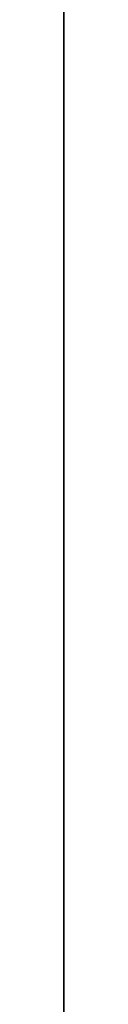
# Model space of a CAD drawing. Units: inches. Extents: x 2083 to 3317, y 1141 to 2115.
# Tile 40 of 256: x 2235.9598 to 2235.9598, y 1477.926 to 1478.1958. Entities that reach past the tile are written whole.
import ezdxf

# ---------------------------------------------------------------- set-up
doc = ezdxf.new("R2010")
doc.units = ezdxf.units.IN
doc.layers.add('A-ANNO-DIMS', color=2, linetype='Continuous', lineweight=18)
doc.layers.add('A-WALL', color=7, linetype='Continuous', lineweight=35)
doc.layers.add('A-WALL-PATT', color=251, linetype='Continuous', lineweight=13, true_color=0x636466)
doc.styles.get("Standard").update_dxf_attribs({"font": 'arial.ttf'})
doc.dimstyles.new('ISO-25', dxfattribs={"dimtxt": 12, "dimasz": 12, "dimexe": 1.25, "dimexo": 0.625, "dimtad": 1, "dimlunit": 3, "dimtxsty": 'Standard', "dimcen": 2.5, "dimadec": 0, "dimazin": 0, "dimtfac": 1, "dimtmove": 0, "dimatfit": 3, "dimfxl": 1, "dimarcsym": 0})

# ---------------------------------------------------------------- blocks, each defined once
blk = doc.blocks.new('*D30')
at = {"layer": 'A-ANNO-DIMS', "color": 0, "lineweight": -2, "transparency": 16777216}
for p, q in [((2240.01786, 1445.27381), (2240.01786, 1448.04553)), ((2254.32933, 1445.27381), (2254.32933, 1448.04553)), ((2228.01786, 1446.79553), (2216.01786, 1446.79553)), ((2240.01786, 1446.79553), (2254.32933, 1446.79553)), ((2266.32933, 1446.79553), (2413.76487, 1446.79553))]:
    blk.add_line(p, q, dxfattribs=at)
at = {"layer": 'A-ANNO-DIMS', "color": 0, "transparency": 16777216}
for points in [[(2228.01786, 1448.79553), (2228.01786, 1444.79553), (2240.01786, 1446.79553)], [(2266.32933, 1448.79553), (2266.32933, 1444.79553), (2254.32933, 1446.79553)]]:
    blk.add_solid(points, dxfattribs=at)
at = {"layer": 'Defpoints', "color": 0, "transparency": 16777216}
for p in [(2254.32933, 1446.79553), (2240.01786, 1444.64881), (2254.32933, 1444.64881)]:
    blk.add_point(p, dxfattribs=at)
at = {"layer": 'A-ANNO-DIMS', "color": 0, "transparency": 16777216, "insert": (2346.0471, 1453.62517), "char_height": 12, "attachment_point": 5}
blk.add_mtext('WC 1\'-2 1/2" TYP.', dxfattribs=at)
blk = doc.blocks.new('*D31')
at = {"layer": 'A-ANNO-DIMS', "color": 0, "lineweight": -2, "transparency": 16777216}
for p, q in [((2237.87114, 1456.64881), (2237.87114, 1541.91518)), ((2239.39286, 1444.64881), (2236.62114, 1444.64881)), ((2237.87114, 1431.54754), (2237.87114, 1444.64881)), ((2239.39286, 1431.54754), (2236.62114, 1431.54754)), ((2237.87114, 1419.54754), (2237.87114, 1407.54754))]:
    blk.add_line(p, q, dxfattribs=at)
at = {"layer": 'A-ANNO-DIMS', "color": 0, "transparency": 16777216}
for points in [[(2235.87114, 1456.64881), (2239.87114, 1456.64881), (2237.87114, 1444.64881)], [(2235.87114, 1419.54754), (2239.87114, 1419.54754), (2237.87114, 1431.54754)]]:
    blk.add_solid(points, dxfattribs=at)
at = {"layer": 'Defpoints', "color": 0, "transparency": 16777216}
for p in [(2237.87114, 1444.64881), (2240.01786, 1444.64881), (2240.01786, 1431.54754)]:
    blk.add_point(p, dxfattribs=at)
at = {"layer": 'A-ANNO-DIMS', "color": 0, "transparency": 16777216, "insert": (2231.21749, 1505.28199), "char_height": 12, "attachment_point": 5, "rotation": 90}
blk.add_mtext('1\'-1" TYP.', dxfattribs=at)
blk = doc.blocks.new('*D45')
at = {"layer": 'A-ANNO-DIMS', "color": 0, "lineweight": -2, "transparency": 16777216}
for p, q in [((2235.95978, 1478.38636), (2235.95978, 1531.36136)), ((2418.95978, 1478.38636), (2418.95978, 1531.36136)), ((2247.95978, 1530.11136), (2406.95978, 1530.11136))]:
    blk.add_line(p, q, dxfattribs=at)
at = {"layer": 'A-ANNO-DIMS', "color": 0, "transparency": 16777216}
for points in [[(2247.95978, 1532.11136), (2247.95978, 1528.11136), (2235.95978, 1530.11136)], [(2406.95978, 1532.11136), (2406.95978, 1528.11136), (2418.95978, 1530.11136)]]:
    blk.add_solid(points, dxfattribs=at)
at = {"layer": 'Defpoints', "color": 0, "transparency": 16777216}
for p in [(2418.95978, 1530.11136), (2235.95978, 1477.76136), (2418.95978, 1477.76136)]:
    blk.add_point(p, dxfattribs=at)
at = {"layer": 'A-ANNO-DIMS', "color": 0, "transparency": 16777216, "insert": (2327.45978, 1536.86733), "char_height": 12, "attachment_point": 5}
blk.add_mtext('15\'-3"', dxfattribs=at)
blk = doc.blocks.new('*D62')
at = {"layer": 'A-ANNO-DIMS', "color": 0, "lineweight": -2, "transparency": 16777216}
for p, q in [((2235.95978, 1469.38636), (2235.95978, 1522.36136)), ((2379.95978, 1469.38636), (2379.95978, 1522.36136)), ((2247.95978, 1521.11136), (2367.95978, 1521.11136))]:
    blk.add_line(p, q, dxfattribs=at)
at = {"layer": 'A-ANNO-DIMS', "color": 0, "transparency": 16777216}
for points in [[(2247.95978, 1523.11136), (2247.95978, 1519.11136), (2235.95978, 1521.11136)], [(2367.95978, 1523.11136), (2367.95978, 1519.11136), (2379.95978, 1521.11136)]]:
    blk.add_solid(points, dxfattribs=at)
at = {"layer": 'Defpoints', "color": 0, "transparency": 16777216}
for p in [(2379.95978, 1521.11136), (2235.95978, 1468.76136), (2379.95978, 1468.76136)]:
    blk.add_point(p, dxfattribs=at)
at = {"layer": 'A-ANNO-DIMS', "color": 0, "transparency": 16777216, "insert": (2307.95978, 1527.86324), "char_height": 12, "attachment_point": 5}
blk.add_mtext('12\'-0"', dxfattribs=at)

msp = doc.modelspace()

# ---------------------------------------------------------------- hatches: boundary and pattern name
at = {"layer": 'A-WALL-PATT'}
h = msp.add_hatch(color=256, dxfattribs=at)
h.dxf.hatch_style = 1
h.paths.add_polyline_path([(3126.95978, 2020.76136), (2748.95978, 2020.76136), (2604.95978, 2020.76136), (2226.95978, 2020.76136), (2226.95978, 1702.76136), (2466.95978, 1702.76136), (2466.95978, 1582.76136), (2418.95978, 1582.76136), (2418.95978, 1477.76136), (2226.95978, 1477.76136), (2226.95978, 1263.26136), (2544.95978, 1263.26136), (2544.95978, 1411.76136), (2604.95978, 1411.76136), (2685.95978, 1411.76136), (2685.95978, 1420.76136), (2604.95978, 1420.76136), (2604.95978, 1573.76136), (2604.95978, 1702.76136), (2604.95978, 2011.76136), (2748.95978, 2011.76136), (2748.95978, 1702.76136), (2862.95978, 1702.76136), (2862.95978, 1621.76136), (2871.95978, 1621.76136), (2871.95978, 1702.76136), (2883.95978, 1702.76136), (2883.95978, 1706.93946, -0.026459), (2883.95978, 1711.76136), (2757.95978, 1711.76136), (2757.95978, 1807.76136), (2787.95978, 1807.76136), (2787.95978, 1812.26136), (2757.95978, 1812.26136), (2757.95978, 2011.76136), (2877.95978, 2011.76136), (2877.95978, 1812.26136), (2847.95978, 1812.26136), (2847.95978, 1807.76136), (2889.83574, 1807.76136), (2889.83574, 1812.26136), (2882.45978, 1812.26136), (2882.45978, 2011.76136), (3117.95978, 2011.76136), (3117.95978, 1812.26136), (2937.83574, 1812.26136), (2937.83574, 1807.76136), (2995.70978, 1807.76136), (2995.70978, 1796.11767), (3000.20978, 1796.11767), (3000.20978, 1807.76136), (3117.95978, 1807.76136), (3117.95978, 1711.76136), (3000.20978, 1711.76136), (3000.20978, 1760.11767), (2998.5727, 1760.11767, -0.020711), (2995.70978, 1760.11767), (2995.70978, 1711.76136), (2931.95978, 1711.76136), (2931.95978, 1702.76136), (3126.95978, 1702.76136)])
h.paths.add_polyline_path([(2471.45978, 2011.76136), (2471.45978, 1810.01136), (2462.71694, 1810.01136), (2462.71694, 1805.51136), (2505.95978, 1805.51136), (2505.95978, 1810.01136), (2475.95978, 1810.01136), (2475.95978, 2011.76136), (2595.95978, 2011.76136), (2595.95978, 1810.01136), (2565.95978, 1810.01136), (2565.95978, 1805.51136), (2595.95978, 1805.51136), (2595.95978, 1711.76136), (2235.95978, 1711.76136), (2235.95978, 1805.51136), (2353.70978, 1805.51136), (2353.70978, 1796.05416), (2358.20978, 1796.05416), (2358.20978, 1805.51136), (2414.71694, 1805.51136), (2414.71694, 1810.01136), (2235.95978, 1810.01136), (2235.95978, 2011.76136)], flags=16)
h.paths.add_polyline_path([(2270.20473, 1994.61001), (2270.20473, 1970.61001), (2246.20473, 1970.61001), (2246.20473, 1994.61001)], flags=0)
edge = h.paths.add_edge_path(flags=0)
edge.add_ellipse((2332.02739, 1899.79818), major_axis=(-3.04299, 3.04299), ratio=0.1682525, start_angle=-161.33217, end_angle=-156.30711, ccw=False)
edge.add_ellipse((2333.08204, 1898.74353), major_axis=(-1.05465, 1.05465), ratio=0.4535321, start_angle=-123.37102, end_angle=-94.15911)
edge = h.paths.add_edge_path(flags=0)
edge.add_ellipse((2332.02739, 1968.87629), major_axis=(3.04299, 3.04299), ratio=0.1682525, start_angle=18.66783, end_angle=23.69289)
edge.add_spline(control_points=[(2332.9256, 1970.6911), (2332.22677, 1970.3361), (2330.89371, 1969.65891), (2328.41308, 1970.93214), (2327.20393, 1967.74871), (2324.7096, 1969.95559), (2322.53282, 1967.01235), (2320.01285, 1971.29581), (2317.68031, 1968.15784), (2316.04053, 1967.10205), (2315.4269, 1966.8096)], knot_values=[0, 0, 0, 0, 2.267059, 4.324559, 6.685584, 8.878641, 11.121502, 14.300359, 17.755284, 19.732645, 19.732645, 19.732645, 19.732645], degree=3, periodic=0)
edge.add_ellipse((2332.02739, 1968.87629), major_axis=(3.04299, 3.04299), ratio=0.1682525, start_angle=18.66783, end_angle=23.69289, ccw=False)
edge.add_ellipse((2333.08204, 1969.93094), major_axis=(1.05465, 1.05465), ratio=0.4535321, start_angle=56.62898, end_angle=85.84089, ccw=False)
edge = h.paths.add_edge_path(flags=0)
edge.add_spline(control_points=[(2296.42829, 1967.98791), (2293.6278, 1965.33631), (2287.70362, 1959.72709), (2299.74386, 1949.9957), (2294.53259, 1935.66853), (2290.57323, 1920.60351), (2293.39412, 1909.97369), (2296.18541, 1904.96654)], knot_values=[0.099185, 0.099185, 0.099185, 0.099185, 0.345301, 0.619822, 0.982653, 1.386093, 1.810555, 1.810555, 1.810555, 1.810555], degree=3, periodic=0)
edge.add_spline(control_points=[(2296.18541, 1904.96654), (2297.38358, 1902.6193), (2298.00097, 1901.94931), (2298.55297, 1901.46815)], knot_values=[0.006246, 0.006246, 0.006246, 0.006246, 0.055476, 0.055476, 0.055476, 0.055476], degree=3, periodic=0)
edge.add_spline(control_points=[(2298.55297, 1901.46815), (2297.25861, 1900.92322), (2295.22529, 1900.23213), (2293.06023, 1900.61421), (2292.10142, 1900.78841), (2292.08958, 1900.79057)], knot_values=[0.312835, 0.312835, 0.312835, 0.312835, 0.40178, 0.474987, 0.475903, 0.475903, 0.475903, 0.475903], degree=3, periodic=0)
edge.add_arc((2292.79365, 1904.66411), 3.93701, 215.4209, 259.69818, ccw=False)
edge.add_spline(control_points=[(2289.58531, 1902.3823), (2289.47665, 1902.53509), (2289.36848, 1902.68804), (2289.26086, 1902.84117)], knot_values=[0.102872, 0.102872, 0.102872, 0.102872, 0.116896, 0.116896, 0.116896, 0.116896], degree=3, periodic=0)
edge.add_spline(control_points=[(2289.26086, 1902.84117), (2288.6866, 1902.55019), (2287.64005, 1902.0199), (2285.88134, 1901.87395), (2283.85297, 1901.50435), (2281.71999, 1899.71054), (2278.46699, 1899.49294), (2276.15714, 1901.8832), (2272.25895, 1899.80407), (2267.77761, 1901.84318), (2262.24388, 1900.18403), (2257.41493, 1901.78206), (2254.31837, 1900.72612), (2253.17828, 1900.33734)], knot_values=[0, 0, 0, 0, 1.907977, 3.477176, 5.261074, 7.972851, 11.680248, 13.717921, 16.939592, 22.789562, 27.502503, 33.595215, 37.145618, 37.145618, 37.145618, 37.145618], degree=3, periodic=0)
edge.add_line((2253.17828, 1900.33734), (2250.24424, 1902.84117))
edge.add_line((2250.24424, 1902.84117), (2250.24424, 1965.8333))
edge.add_line((2250.24424, 1965.8333), (2253.17828, 1968.33712))
edge.add_spline(control_points=[(2253.17828, 1968.33712), (2254.31837, 1967.94835), (2257.41493, 1966.89241), (2262.24388, 1968.49043), (2267.77761, 1966.83128), (2271.52673, 1968.53722), (2273.87591, 1967.82829), (2274.2067, 1967.72764)], knot_values=[0, 0, 0, 0, 0.09018, 0.244935, 0.364644, 0.513233, 0.537855, 0.537855, 0.537855, 0.537855], degree=3, periodic=0)
edge.add_arc((2274.35289, 1963.79335), 3.93701, 72.05113, 92.12795, ccw=False)
edge.add_arc((2281.29693, 1985.23), 18.5963, 252.051134, 288.565722)
edge.add_arc((2292.31672, 1956.02888), 12.64608, 71.026788, 113.778218, ccw=False)
edge = h.paths.add_edge_path(flags=0)
edge.add_spline(control_points=[(2274.89941, 1951.85619), (2275.06616, 1951.61659), (2275.23269, 1951.37659), (2275.39799, 1951.13585)], knot_values=[1.409916, 1.409916, 1.409916, 1.409916, 1.43159, 1.43159, 1.43159, 1.43159], degree=3, periodic=0)
edge.add_spline(control_points=[(2275.39799, 1951.13585), (2275.79211, 1950.56189), (2276.17923, 1949.98377), (2276.54555, 1949.3971)], knot_values=[1.358238, 1.358238, 1.358238, 1.358238, 1.409916, 1.409916, 1.409916, 1.409916], degree=3, periodic=0)
edge.add_line((2276.54555, 1949.3971), (2277.43729, 1947.86218))
edge.add_spline(control_points=[(2277.43729, 1947.86218), (2276.30383, 1945.67311), (2274.6397, 1942.42688), (2274.63161, 1938.0939), (2272.79912, 1930.85155), (2274.35643, 1943.89705), (2275.94768, 1947.92336), (2276.54555, 1949.3971)], knot_values=[0.005632, 0.005632, 0.005632, 0.005632, 0.186014, 0.266002, 0.357087, 0.59639, 0.739732, 0.739732, 0.739732, 0.739732], degree=3, periodic=0)
edge.add_spline(control_points=[(2276.54555, 1949.3971), (2276.17923, 1949.98377), (2275.79211, 1950.56189), (2275.39799, 1951.13585)], knot_values=[1.358238, 1.358238, 1.358238, 1.358238, 1.409916, 1.409916, 1.409916, 1.409916], degree=3, periodic=0)
edge.add_spline(control_points=[(2275.39799, 1951.13585), (2274.9425, 1950.08045), (2274.20776, 1948.02527), (2273.9346, 1944.85148), (2272.46853, 1937.62749), (2273.46622, 1945.69647), (2274.70062, 1951.05947), (2274.89941, 1951.85619)], knot_values=[0.104364, 0.104364, 0.104364, 0.104364, 0.189636, 0.269624, 0.36071, 0.600013, 0.644622, 0.644622, 0.644622, 0.644622], degree=3, periodic=0)
h.paths.add_polyline_path([(2269.16751, 1963.12757, -0.357527), (2268.17063, 1960.97637, -0.092561), (2268.17063, 1939.43632, -0.357527), (2269.16751, 1937.28512, -0.357527), (2267.01631, 1938.282, -0.164785), (2254.68558, 1938.282, -0.357527), (2252.53438, 1937.28512, -0.357527), (2253.53126, 1939.43632, -0.092561), (2253.53126, 1960.97637, -0.357527), (2252.53438, 1963.12757, -0.357527), (2254.68558, 1962.13069, -0.164785), (2267.01631, 1962.13069, -0.357527)], flags=0)
h.paths.add_polyline_path([(2248.87407, 1967.8018), (2248.87407, 1957.02771), (2249.45778, 1957.02771), (2249.45778, 1911.64676), (2248.87407, 1911.64676), (2248.87407, 1900.87267), (2246.51186, 1900.87267, 0.197327), (2244.14966, 1902.45687), (2244.14966, 1966.21759, 0.197327), (2246.51186, 1967.8018)], flags=0)
h.paths.add_polyline_path([(2269.16751, 1931.38934, -0.357527), (2268.17063, 1929.23814, -0.092561), (2268.17063, 1907.6981, -0.357527), (2269.16751, 1905.54689, -0.357527), (2267.01631, 1906.54377, -0.164785), (2254.68558, 1906.54377, -0.357527), (2252.53438, 1905.54689, -0.357527), (2253.53126, 1907.6981, -0.092561), (2253.53126, 1929.23814, -0.357527), (2252.53438, 1931.38934, -0.357527), (2254.68558, 1930.39246, -0.164785), (2267.01631, 1930.39246, -0.357527)], flags=0)
edge = h.paths.add_edge_path(flags=0)
edge.add_spline(control_points=[(2276.19686, 1906.7237), (2276.16814, 1909.02893), (2276.11405, 1913.37185), (2270.59842, 1924.92498), (2273.90517, 1919.01278), (2275.92171, 1916.26206), (2275.47457, 1912.40215), (2277.25787, 1910.38062), (2276.69604, 1908.22504), (2276.64622, 1906.81302), (2276.61782, 1906.00841)], knot_values=[0, 0, 0, 0, 8.61026, 16.221274, 18.843057, 23.804898, 27.440828, 29.356102, 31.203478, 33.650687, 33.650687, 33.650687, 33.650687], degree=3, periodic=0)
edge.add_spline(control_points=[(2276.61782, 1906.00841), (2276.62331, 1905.62414), (2276.49774, 1904.62866), (2275.44178, 1903.85473), (2274.93731, 1903.08045), (2274.85908, 1902.84117)], knot_values=[0.156488, 0.156488, 0.156488, 0.156488, 0.184398, 0.231376, 0.250598, 0.250598, 0.250598, 0.250598], degree=3, periodic=0)
edge.add_line((2274.85908, 1902.84117), (2276.50598, 1902.84117))
edge.add_spline(control_points=[(2276.50598, 1902.84117), (2276.78831, 1903.08494), (2277.66507, 1904.1252), (2278.24954, 1904.34074), (2277.65387, 1908.52739), (2278.15567, 1906.22781), (2278.10046, 1905.28595), (2278.84667, 1904.06901), (2277.85679, 1903.41495), (2277.87419, 1902.99105), (2277.90356, 1902.84117)], knot_values=[0.059574, 0.059574, 0.059574, 0.059574, 0.080753, 0.103741, 0.16972, 0.176036, 0.207137, 0.240474, 0.262341, 0.27366, 0.27366, 0.27366, 0.27366], degree=3, periodic=0)
edge.add_line((2277.90356, 1902.84117), (2280.02983, 1902.84117))
edge.add_spline(control_points=[(2280.02983, 1902.84117), (2279.88822, 1903.0884), (2279.49926, 1903.98155), (2280.15228, 1905.93935), (2278.10362, 1909.65776), (2279.76239, 1907.18529), (2280.3279, 1904.87486), (2280.48511, 1903.48959), (2281.46327, 1903.24943), (2281.75834, 1902.9365), (2281.83404, 1902.84117)], knot_values=[0.013856, 0.013856, 0.013856, 0.013856, 0.034874, 0.088867, 0.107879, 0.126738, 0.158714, 0.193757, 0.217487, 0.226722, 0.226722, 0.226722, 0.226722], degree=3, periodic=0)
edge.add_spline(control_points=[(2281.83404, 1902.84117), (2281.78753, 1902.8267), (2281.64702, 1902.78299), (2281.39553, 1902.85949), (2281.08808, 1902.98524), (2280.72068, 1903.0609), (2280.33345, 1903.02573), (2280.12477, 1902.89888), (2280.02983, 1902.84117)], knot_values=[0, 0, 0, 0, 0.14413, 0.435517, 0.749276, 1.153046, 1.548371, 1.878348, 1.878348, 1.878348, 1.878348], degree=3, periodic=0)
edge.add_line((2280.02983, 1902.84117), (2277.90356, 1902.84117))
edge.add_spline(control_points=[(2277.90356, 1902.84117), (2277.89286, 1902.79586), (2277.8654, 1902.67964), (2277.60748, 1902.68748), (2277.27405, 1902.8007), (2276.83792, 1902.61977), (2276.58381, 1902.78926), (2276.50598, 1902.84117)], knot_values=[0, 0, 0, 0, 0.127189, 0.326199, 0.628009, 1.24357, 1.515331, 1.515331, 1.515331, 1.515331], degree=3, periodic=0)
edge.add_line((2276.50598, 1902.84117), (2274.85908, 1902.84117))
edge.add_spline(control_points=[(2274.85908, 1902.84117), (2274.81444, 1902.89859), (2274.72513, 1903.01345), (2274.49348, 1903.11897), (2274.24429, 1902.96054), (2273.93712, 1903.18494), (2273.61404, 1902.98314), (2273.40832, 1902.88304), (2273.32225, 1902.84117)], knot_values=[0, 0, 0, 0, 0.21843, 0.436957, 0.687977, 0.990379, 1.398396, 1.69185, 1.69185, 1.69185, 1.69185], degree=3, periodic=0)
edge.add_spline(control_points=[(2273.32225, 1902.84117), (2273.61674, 1903.44569), (2274.274, 1904.53825), (2276.02724, 1904.5737), (2276.20696, 1906.58364), (2276.19686, 1906.7237)], knot_values=[0.012227, 0.012227, 0.012227, 0.012227, 0.059472, 0.106218, 0.134458, 0.134458, 0.134458, 0.134458], degree=3, periodic=0)
h.paths.add_polyline_path([(2270.77605, 1897.78983), (2270.77605, 1873.78983), (2246.77605, 1873.78983), (2246.77605, 1897.78983)], flags=0)
h.paths.add_polyline_path([(2353.70978, 1760.00506), (2353.70978, 1760.05416), (2358.20978, 1760.05416, -0.033729)], flags=0)
h.paths.add_polyline_path([(2321.81912, 1737.52919), (2341.99533, 1737.52919, -0.414214), (2343.20327, 1736.32124), (2343.20327, 1721.0206, -0.414214), (2341.99533, 1719.81265), (2321.81912, 1719.81265, -0.414214), (2320.61117, 1721.0206), (2320.61117, 1736.32124, -0.414214)], flags=0)
h.paths.add_polyline_path([(2324.23501, 1736.32124), (2339.57944, 1736.32124, -0.414214), (2341.99533, 1733.90535), (2341.99533, 1725.44973, -0.414214), (2339.57944, 1723.03384), (2333.68059, 1723.03384), (2333.84532, 1722.04547, -0.870646), (2335.4254, 1721.82589, -0.767327), (2333.92269, 1721.42324), (2331.29102, 1721.42324, -0.767327), (2329.78832, 1721.82589, -0.870646), (2331.3684, 1722.04547), (2331.53313, 1723.03384), (2324.23501, 1723.03384, -0.414214), (2321.81912, 1725.44973), (2321.81912, 1733.90535, -0.414214)], flags=0)
h.paths.add_polyline_path([(2570.48379, 1928.61544), (2589.68379, 1928.61544), (2590.16883, 1928.61544), (2590.16883, 1904.9934), (2570.48379, 1904.9934)], flags=0)
h.paths.add_polyline_path([(2574.44732, 1927.26382, -1), (2572.82884, 1927.26382, -1)], flags=0)
h.paths.add_polyline_path([(2573.08987, 1926.94088), (2573.92503, 1927.77604), (2574.14774, 1927.55333), (2573.31258, 1926.71817)], flags=0)
h.paths.add_polyline_path([(2578.77906, 1919.72962, -1), (2571.59166, 1919.72962, -1)], flags=0)
h.paths.add_polyline_path([(2578.38536, 1919.72962, -1), (2571.98536, 1919.72962, -1)], flags=0)
h.paths.add_polyline_path([(2331.59576, 1729.47622, -1), (2333.61795, 1729.47622, -1)], flags=0)
h.paths.add_polyline_path([(2578.03423, 1927.26382, -1), (2576.41574, 1927.26382, -1)], flags=0)
h.paths.add_polyline_path([(2576.68885, 1927.53109), (2576.91156, 1927.7538), (2577.74673, 1926.91863), (2577.52402, 1926.69592)], flags=0)
h.paths.add_polyline_path([(2578.13906, 1909.85954, -1), (2572.23166, 1909.85954, -1)], flags=0)
h.paths.add_polyline_path([(2577.74536, 1909.85954, -1), (2572.62536, 1909.85954, -1)], flags=0)
h.paths.add_polyline_path([(2583.79772, 1927.26382, -1), (2582.17923, 1927.26382, -1)], flags=0)
h.paths.add_polyline_path([(2582.71865, 1927.7538), (2583.55381, 1926.91863), (2583.3311, 1926.69592), (2582.49594, 1927.53109)], flags=0)
h.paths.add_polyline_path([(2582.49594, 1927.53109), (2582.71865, 1927.7538), (2583.55381, 1926.91863), (2583.3311, 1926.69592)], flags=0)
h.paths.add_polyline_path([(2587.73906, 1920.52962, -1), (2581.83166, 1920.52962, -1)], flags=0)
h.paths.add_polyline_path([(2587.34536, 1920.52962, -1), (2582.22536, 1920.52962, -1)], flags=0)
h.paths.add_polyline_path([(2587.38462, 1927.26382, -1), (2585.76613, 1927.26382, -1)], flags=0)
h.paths.add_polyline_path([(2586.08199, 1926.98025), (2586.91716, 1927.81541), (2587.13987, 1927.5927), (2586.3047, 1926.75754)], flags=0)
h.paths.add_polyline_path([(2588.37906, 1910.65954, -1), (2581.19166, 1910.65954, -1)], flags=0)
h.paths.add_polyline_path([(2587.98536, 1910.65954, -1), (2581.58536, 1910.65954, -1)], flags=0)
h.paths.add_polyline_path([(2417.16773, 1729.4779), (2437.34394, 1729.4779, -0.414214), (2438.55188, 1728.26995), (2438.55188, 1712.96931, -0.414214), (2437.34394, 1711.76136), (2417.16773, 1711.76136, -0.414214), (2415.95978, 1712.96931), (2415.95978, 1728.26995, -0.414214)], flags=0)
h.paths.add_polyline_path([(2419.58362, 1728.26995), (2434.92805, 1728.26995, -0.414214), (2437.34394, 1725.85406), (2437.34394, 1717.39844, -0.414214), (2434.92805, 1714.98255), (2429.0292, 1714.98255), (2429.19393, 1713.99418, -0.870646), (2430.77401, 1713.7746, -0.767327), (2429.2713, 1713.37195), (2426.63963, 1713.37195, -0.767327), (2425.13693, 1713.7746, -0.870646), (2426.71701, 1713.99418), (2426.88174, 1714.98255), (2419.58362, 1714.98255, -0.414214), (2417.16773, 1717.39844), (2417.16773, 1725.85406, -0.414214)], flags=0)
h.paths.add_polyline_path([(2419.58362, 1728.26995), (2434.92805, 1728.26995, -0.414214), (2437.34394, 1725.85406), (2437.34394, 1717.39844, -0.414214), (2434.92805, 1714.98255), (2429.0292, 1714.98255), (2428.35812, 1719.00903), (2427.55282, 1719.00903), (2426.88174, 1714.98255), (2419.58362, 1714.98255, -0.414214), (2417.16773, 1717.39844), (2417.16773, 1725.85406, -0.414214)], flags=0)
h.paths.add_polyline_path([(2426.94437, 1721.42492, -1), (2428.96656, 1721.42492, -1)], flags=0)
h.paths.add_polyline_path([(2475.95978, 1702.76136), (2595.95978, 1702.76136), (2595.95978, 1582.76136), (2475.95978, 1582.76136)], flags=16)
h.paths.add_polyline_path([(2427.95978, 1573.76136), (2595.95978, 1573.76136), (2595.95978, 1468.76136), (2595.95978, 1420.76136), (2384.45978, 1420.76136), (2384.45978, 1468.76136), (2427.95978, 1468.76136)], flags=16)
h.paths.add_polyline_path([(2379.95978, 1468.76136), (2379.95978, 1420.76136), (2235.95978, 1420.76136), (2235.95978, 1468.76136)], flags=16)
h.paths.add_polyline_path([(2317.816, 1466.69577), (2337.9922, 1466.69577, -0.414214), (2339.20015, 1465.48782), (2339.20015, 1450.18718, -0.414214), (2337.9922, 1448.97923), (2317.816, 1448.97923, -0.414214), (2316.60805, 1450.18718), (2316.60805, 1465.48782, -0.414214)], flags=0)
h.paths.add_polyline_path([(2320.23189, 1465.48782), (2335.57631, 1465.48782, -0.414214), (2337.9922, 1463.07193), (2337.9922, 1454.61631, -0.414214), (2335.57631, 1452.20042), (2329.67747, 1452.20042), (2329.84219, 1451.21205, -0.870646), (2331.42228, 1450.99247, -0.767327), (2329.91957, 1450.58983), (2327.2879, 1450.58983, -0.767327), (2325.7852, 1450.99247, -0.870646), (2327.36528, 1451.21205), (2327.53001, 1452.20042), (2320.23189, 1452.20042, -0.414214), (2317.816, 1454.61631), (2317.816, 1463.07193, -0.414214)], flags=0)
h.paths.add_polyline_path([(2320.23189, 1465.48782), (2335.57631, 1465.48782, -0.414214), (2337.9922, 1463.07193), (2337.9922, 1454.61631, -0.414214), (2335.57631, 1452.20042), (2329.67747, 1452.20042), (2329.00638, 1456.22691), (2328.20109, 1456.22691), (2327.53001, 1452.20042), (2320.23189, 1452.20042, -0.414214), (2317.816, 1454.61631), (2317.816, 1463.07193, -0.414214)], flags=0)
h.paths.add_polyline_path([(2327.59264, 1458.6428, -1), (2329.61483, 1458.6428, -1)], flags=0)
h.paths.add_polyline_path([(2244.41174, 1433.34045), (2241.92094, 1433.34045, -0.414214), (2240.01786, 1435.24354), (2240.01786, 1440.95281, -0.414211), (2241.92093, 1442.8559), (2244.41174, 1442.8559, -1.976472)], flags=0)
h.paths.add_polyline_path([(2245.35689, 1434.39754, -0.414214), (2245.35689, 1441.79881, -2.144098)], flags=0)
h.paths.add_polyline_path([(2535.95978, 1416.26136), (2535.95978, 1272.26136), (2235.95978, 1272.26136), (2235.95978, 1416.26136)], flags=16)
h.paths.add_polyline_path([(2260.11956, 1384.29284), (2260.11956, 1362.03865), (2237.86537, 1362.03865), (2237.86537, 1384.29284)], flags=0)
edge = h.paths.add_edge_path(flags=0)
edge.add_line((2318.25185, 1362.0933), (2318.1458, 1362.00097))
edge.add_ellipse((2317.44512, 1360.43104), major_axis=(2.82164, 2.82164), ratio=0.1682525, start_angle=18.66783, end_angle=20.94813, ccw=False)
edge.add_ellipse((2318.42305, 1361.40897), major_axis=(0.97793, 0.97793), ratio=0.4535321, start_angle=56.62898, end_angle=70.2262, ccw=False)
edge = h.paths.add_edge_path(flags=0)
edge.add_line((2319.10737, 1295.57108), (2319.01504, 1295.67713))
edge.add_ellipse((2317.44512, 1296.37781), major_axis=(-2.82164, 2.82164), ratio=0.1682525, start_angle=-161.33217, end_angle=-159.05187, ccw=False)
edge.add_ellipse((2318.42305, 1295.39988), major_axis=(-0.97793, 0.97793), ratio=0.4535321, start_angle=-123.37102, end_angle=-109.7738)
edge = h.paths.add_edge_path(flags=0)
edge.add_spline(control_points=[(2284.21035, 1301.17022), (2284.58069, 1300.44472), (2284.89119, 1299.89202), (2285.15955, 1299.46102)], knot_values=[0.039066, 0.039066, 0.039066, 0.039066, 0.055476, 0.055476, 0.055476, 0.055476], degree=3, periodic=0)
edge.add_line((2285.15955, 1299.46102), (2284.21035, 1301.17022))
edge = h.paths.add_edge_path(flags=0)
edge.add_line((2280.41246, 1297.29801), (2283.36999, 1297.03612))
edge.add_line((2283.36999, 1297.03612), (2286.40569, 1297.92631))
edge.add_spline(control_points=[(2286.40569, 1297.92631), (2285.30549, 1297.46312), (2284.34478, 1297.12915), (2283.36999, 1297.03612)], knot_values=[0.394369, 0.394369, 0.394369, 0.394369, 0.475903, 0.475903, 0.475903, 0.475903], degree=3, periodic=0)
edge.add_spline(control_points=[(2283.36999, 1297.03612), (2283.28139, 1297.02767), (2282.31629, 1296.95734), (2281.3125, 1297.13448), (2280.42344, 1297.29602), (2280.41246, 1297.29801)], knot_values=[0.312835, 0.312835, 0.312835, 0.312835, 0.320246, 0.393453, 0.394369, 0.394369, 0.394369, 0.394369], degree=3, periodic=0)
edge = h.paths.add_edge_path(flags=0)
edge.add_line((2284.43556, 1359.60729), (2280.44629, 1355.32805))
edge.add_line((2280.44629, 1355.32805), (2279.57999, 1351.01775))
edge.add_line((2279.57999, 1351.01775), (2282.41297, 1346.58043))
edge.add_spline(control_points=[(2282.41297, 1346.58043), (2283.15333, 1345.58924), (2284.2529, 1344.0289), (2284.80104, 1342.38717), (2284.93516, 1341.80554)], knot_values=[1.240098, 1.240098, 1.240098, 1.240098, 1.332892, 1.382712, 1.382712, 1.382712, 1.382712], degree=3, periodic=0)
edge.add_spline(control_points=[(2284.93516, 1341.80554), (2285.31911, 1340.1406), (2285.23303, 1338.4092), (2284.90994, 1336.65412)], knot_values=[1.097484, 1.097484, 1.097484, 1.097484, 1.240098, 1.240098, 1.240098, 1.240098], degree=3, periodic=0)
edge.add_spline(control_points=[(2284.90994, 1336.65412), (2284.58685, 1334.89904), (2284.02675, 1333.12027), (2283.46264, 1331.36058)], knot_values=[0.95487, 0.95487, 0.95487, 0.95487, 1.097484, 1.097484, 1.097484, 1.097484], degree=3, periodic=0)
edge.add_line((2283.46264, 1331.36058), (2281.89038, 1326.15336))
edge.add_line((2281.89038, 1326.15336), (2280.75626, 1321.05609))
edge.add_line((2280.75626, 1321.05609), (2280.2992, 1316.00198))
edge.add_line((2280.2992, 1316.00198), (2280.71593, 1310.95007))
edge.add_line((2280.71593, 1310.95007), (2282.02809, 1305.97214))
edge.add_line((2282.02809, 1305.97214), (2284.21035, 1301.17022))
edge.add_spline(control_points=[(2284.21035, 1301.17022), (2283.34073, 1302.73019), (2282.6119, 1304.33649), (2282.02809, 1305.97214)], knot_values=[0.099185, 0.099185, 0.099185, 0.099185, 0.241799, 0.241799, 0.241799, 0.241799], degree=3, periodic=0)
edge.add_spline(control_points=[(2282.02809, 1305.97214), (2281.44428, 1307.60778), (2281.00549, 1309.27276), (2280.71593, 1310.95007)], knot_values=[0.241799, 0.241799, 0.241799, 0.241799, 0.384413, 0.384413, 0.384413, 0.384413], degree=3, periodic=0)
edge.add_spline(control_points=[(2280.71593, 1310.95007), (2280.43324, 1312.58761), (2280.28939, 1314.27696), (2280.29889, 1315.96203), (2280.2992, 1316.00198)], knot_values=[0.384413, 0.384413, 0.384413, 0.384413, 0.523647, 0.527028, 0.527028, 0.527028, 0.527028], degree=3, periodic=0)
edge.add_spline(control_points=[(2280.2992, 1316.00198), (2280.31233, 1317.68696), (2280.47787, 1319.36793), (2280.75626, 1321.05609)], knot_values=[0.527028, 0.527028, 0.527028, 0.527028, 0.669642, 0.669642, 0.669642, 0.669642], degree=3, periodic=0)
edge.add_spline(control_points=[(2280.75626, 1321.05609), (2281.03465, 1322.74425), (2281.42588, 1324.43961), (2281.89038, 1326.15336)], knot_values=[0.669642, 0.669642, 0.669642, 0.669642, 0.812256, 0.812256, 0.812256, 0.812256], degree=3, periodic=0)
edge.add_spline(control_points=[(2281.89038, 1326.15336), (2282.26438, 1327.53325), (2282.78787, 1329.26181), (2283.35275, 1331.01778), (2283.46264, 1331.36058)], knot_values=[0.812256, 0.812256, 0.812256, 0.812256, 0.927087, 0.95487, 0.95487, 0.95487, 0.95487], degree=3, periodic=0)
edge.add_line((2283.46264, 1331.36058), (2284.90994, 1336.65412))
edge.add_line((2284.90994, 1336.65412), (2284.93516, 1341.80554))
edge.add_line((2284.93516, 1341.80554), (2282.41297, 1346.58043))
edge.add_spline(control_points=[(2282.41297, 1346.58043), (2281.27513, 1348.10379), (2280.07845, 1349.57032), (2279.57999, 1351.01775)], knot_values=[1.382712, 1.382712, 1.382712, 1.382712, 1.525326, 1.525326, 1.525326, 1.525326], degree=3, periodic=0)
edge.add_spline(control_points=[(2279.57999, 1351.01775), (2279.44328, 1351.41472), (2279.13631, 1352.85692), (2279.73519, 1354.29039), (2280.44629, 1355.32805)], knot_values=[1.525326, 1.525326, 1.525326, 1.525326, 1.564439, 1.667941, 1.667941, 1.667941, 1.667941], degree=3, periodic=0)
edge.add_spline(control_points=[(2280.44629, 1355.32805), (2281.42611, 1356.75784), (2282.93084, 1358.18256), (2284.43556, 1359.60729)], knot_values=[1.667941, 1.667941, 1.667941, 1.667941, 1.810555, 1.810555, 1.810555, 1.810555], degree=3, periodic=0)
edge.add_arc((2280.62307, 1348.51818), 11.72618, 71.026788, 113.778218)
edge.add_arc((2270.40489, 1375.59516), 17.24357, 252.051134, 288.565722, ccw=False)
edge.add_arc((2263.96597, 1355.71785), 3.65062, 72.05113, 92.12795)
edge.add_arc((2263.96597, 1355.71785), 3.65062, 92.12795, 177.98513)
edge.add_spline(control_points=[(2260.3176, 1355.8462), (2260.26042, 1354.22067), (2260.55128, 1350.18655), (2262.99934, 1346.76625), (2264.47274, 1344.64902)], knot_values=[1.43159, 1.43159, 1.43159, 1.43159, 1.564144, 1.770695, 1.770695, 1.770695, 1.770695], degree=3, periodic=0)
edge.add_line((2264.47274, 1344.64902), (2264.93559, 1343.98253))
edge.add_spline(control_points=[(2263.80104, 1340.24811), (2263.84324, 1340.51409), (2264.06724, 1341.75647), (2264.51269, 1343.00245), (2264.93505, 1343.98108)], knot_values=[0.53657, 0.53657, 0.53657, 0.53657, 0.559349, 0.644622, 0.644622, 0.644622, 0.644622], degree=3, periodic=0)
edge.add_spline(control_points=[(2264.93505, 1343.98108), (2265.11777, 1343.71497), (2265.29888, 1343.44791), (2265.47676, 1343.17936)], knot_values=[1.384077, 1.384077, 1.384077, 1.384077, 1.409916, 1.409916, 1.409916, 1.409916], degree=3, periodic=0)
edge.add_spline(control_points=[(2265.47676, 1343.17936), (2265.65464, 1342.91082), (2265.8293, 1342.64081), (2265.99913, 1342.36881)], knot_values=[1.358238, 1.358238, 1.358238, 1.358238, 1.384077, 1.384077, 1.384077, 1.384077], degree=3, periodic=0)
edge.add_line((2265.99913, 1342.36881), (2266.82601, 1340.94555))
edge.add_spline(control_points=[(2266.82601, 1340.94555), (2268.8944, 1337.08969), (2271.39817, 1325.843), (2270.51616, 1310.56856), (2275.91938, 1301.86061), (2277.78951, 1299.19945)], knot_values=[0.116896, 0.116896, 0.116896, 0.116896, 0.472987, 1.050969, 1.313793, 1.313793, 1.313793, 1.313793], degree=3, periodic=0)
edge.add_spline(control_points=[(2277.78951, 1299.19945), (2277.83941, 1299.12845), (2277.88943, 1299.0575), (2277.93957, 1298.98658)], knot_values=[0.109884, 0.109884, 0.109884, 0.109884, 0.116896, 0.116896, 0.116896, 0.116896], degree=3, periodic=0)
edge.add_line((2277.93957, 1298.98658), (2277.78885, 1299.19911))
edge.add_spline(control_points=[(2277.78885, 1299.19911), (2277.25658, 1298.92941), (2276.28635, 1298.4379), (2275.03935, 1298.33442), (2274.38333, 1298.2389), (2274.21525, 1298.20934)], knot_values=[33.12187, 33.12187, 33.12187, 33.12187, 35.029056, 36.598255, 37.144827, 37.144827, 37.144827, 37.144827], degree=3, periodic=0)
edge.add_line((2274.21525, 1298.20934), (2273.07315, 1297.89296))
edge.add_spline(control_points=[(2273.07315, 1297.89296), (2272.32294, 1297.57978), (2271.03915, 1296.51051), (2269.24839, 1296.22606), (2268.4231, 1296.37465)], knot_values=[26.532584, 26.532584, 26.532584, 26.532584, 29.198919, 31.839101, 31.839101, 31.839101, 31.839101], degree=3, periodic=0)
edge.add_line((2268.4231, 1296.37465), (2263.8785, 1297.45753))
edge.add_spline(control_points=[(2263.8785, 1297.45753), (2263.55608, 1297.35943), (2261.86031, 1296.83869), (2260.23878, 1297.28241), (2258.93345, 1297.51646)], knot_values=[15.919551, 15.919551, 15.919551, 15.919551, 16.939592, 21.226067, 21.226067, 21.226067, 21.226067], degree=3, periodic=0)
edge.add_line((2258.93345, 1297.51646), (2254.05523, 1297.32901))
edge.add_spline(control_points=[(2254.05523, 1297.32901), (2253.75553, 1297.29582), (2252.11368, 1297.16517), (2250.46187, 1297.54422), (2249.12969, 1297.66788)], knot_values=[5.306517, 5.306517, 5.306517, 5.306517, 6.276435, 10.613034, 10.613034, 10.613034, 10.613034], degree=3, periodic=0)
edge.add_line((2249.12969, 1297.66788), (2244.33165, 1296.87776))
edge.add_line((2244.33165, 1296.87776), (2241.61103, 1299.19945))
edge.add_line((2241.61103, 1299.19945), (2241.61103, 1357.6094))
edge.add_line((2241.61103, 1357.6094), (2244.33165, 1359.9311))
edge.add_line((2244.33165, 1359.9311), (2252.72882, 1359.54269))
edge.add_spline(control_points=[(2252.72882, 1359.54269), (2252.87094, 1359.54644), (2253.30574, 1359.54817), (2253.73984, 1359.51427), (2254.03174, 1359.48243)], knot_values=[0.233291, 0.233291, 0.233291, 0.233291, 0.244935, 0.268927, 0.268927, 0.268927, 0.268927], degree=3, periodic=0)
edge.add_line((2254.03174, 1359.48243), (2259.58719, 1359.41639))
edge.add_spline(control_points=[(2259.58719, 1359.41639), (2260.67707, 1359.6285), (2262.0732, 1359.897), (2263.52369, 1359.45928), (2263.83042, 1359.36595)], knot_values=[0.422516, 0.422516, 0.422516, 0.422516, 0.513233, 0.537855, 0.537855, 0.537855, 0.537855], degree=3, periodic=0)
edge.add_arc((2263.96597, 1355.71785), 3.65062, 72.05113, 92.12795, ccw=False)
edge.add_arc((2270.40489, 1375.59516), 17.24357, 252.051134, 288.565722)
edge.add_arc((2280.62307, 1348.51818), 11.72618, 71.026788, 113.778218, ccw=False)
h.paths.add_polyline_path([(2240.34053, 1359.43471), (2240.34053, 1349.44435), (2240.88178, 1349.44435), (2240.88178, 1307.3645), (2240.34053, 1307.3645), (2240.34053, 1297.37414), (2238.15016, 1297.37414, 0.197327), (2235.95978, 1298.84311), (2235.95978, 1357.96575, 0.197327), (2238.15016, 1359.43471)], flags=0)
h.paths.add_polyline_path([(2259.15779, 1355.1005, -0.357527), (2258.23342, 1353.10578, -0.092561), (2258.23342, 1333.1326, -0.357527), (2259.15779, 1331.13788, -0.357527), (2257.16307, 1332.06225, -0.164785), (2245.7293, 1332.06225, -0.357527), (2243.73458, 1331.13788, -0.357527), (2244.65895, 1333.1326, -0.092561), (2244.65895, 1353.10578, -0.357527), (2243.73458, 1355.1005, -0.357527), (2245.7293, 1354.17613, -0.164785), (2257.16307, 1354.17613, -0.357527)], flags=0)
edge = h.paths.add_edge_path(flags=0)
edge.add_line((2265.99913, 1342.36881), (2266.82601, 1340.94555))
edge.add_line((2266.82601, 1340.94555), (2265.30756, 1337.81407))
edge.add_line((2265.30756, 1337.81407), (2264.35823, 1334.65294))
edge.add_line((2264.35823, 1334.65294), (2264.26201, 1333.7997))
edge.add_spline(control_points=[(2264.26201, 1333.7997), (2264.20836, 1333.18705), (2264.16206, 1332.36553), (2264.00714, 1331.41393), (2263.96905, 1331.20183)], knot_values=[0.464444, 0.464444, 0.464444, 0.464444, 0.516691, 0.531608, 0.531608, 0.531608, 0.531608], degree=3, periodic=0)
edge.add_spline(control_points=[(2263.96905, 1331.20183), (2263.77453, 1330.11887), (2263.42437, 1328.79084), (2263.25742, 1328.53065), (2263.23403, 1328.51461)], knot_values=[0.372682, 0.372682, 0.372682, 0.372682, 0.44885, 0.464444, 0.464444, 0.464444, 0.464444], degree=3, periodic=0)
edge.add_spline(control_points=[(2263.23403, 1328.51461), (2263.09638, 1328.42023), (2263.13117, 1329.30148), (2263.27495, 1330.61575)], knot_values=[0.280919, 0.280919, 0.280919, 0.280919, 0.372682, 0.372682, 0.372682, 0.372682], degree=3, periodic=0)
edge.add_spline(control_points=[(2263.27495, 1330.61575), (2263.41874, 1331.93002), (2263.67152, 1333.67732), (2263.96985, 1335.31503)], knot_values=[0.189157, 0.189157, 0.189157, 0.189157, 0.280919, 0.280919, 0.280919, 0.280919], degree=3, periodic=0)
edge.add_spline(control_points=[(2263.96985, 1335.31503), (2264.1005, 1336.03219), (2264.41878, 1337.62191), (2264.75485, 1338.86443), (2264.94742, 1339.49112)], knot_values=[0.097394, 0.097394, 0.097394, 0.097394, 0.137578, 0.189157, 0.189157, 0.189157, 0.189157], degree=3, periodic=0)
edge.add_spline(control_points=[(2264.94742, 1339.49112), (2265.29002, 1340.60605), (2265.64424, 1341.494), (2265.99913, 1342.36881)], knot_values=[0.005632, 0.005632, 0.005632, 0.005632, 0.097394, 0.097394, 0.097394, 0.097394], degree=3, periodic=0)
h.paths.add_polyline_path([(2259.15779, 1325.67097, -0.357527), (2258.23342, 1323.67625, -0.092561), (2258.23342, 1303.70307, -0.357527), (2259.15779, 1301.70835, -0.357527), (2257.16307, 1302.63272, -0.164785), (2245.7293, 1302.63272, -0.357527), (2243.73458, 1301.70835, -0.357527), (2244.65895, 1303.70307, -0.092561), (2244.65895, 1323.67625, -0.357527), (2243.73458, 1325.67097, -0.357527), (2245.7293, 1324.74661, -0.164785), (2257.16307, 1324.74661, -0.357527)], flags=0)
edge = h.paths.add_edge_path(flags=0)
edge.add_spline(control_points=[(2261.70894, 1317.31142), (2261.67948, 1317.41758), (2261.76186, 1317.38853), (2262.49074, 1316.08987), (2262.96218, 1315.3009)], knot_values=[14.955861, 14.955861, 14.955861, 14.955861, 16.221274, 18.694826, 18.694826, 18.694826, 18.694826], degree=3, periodic=0)
edge.add_spline(control_points=[(2262.96218, 1315.3009), (2262.99044, 1315.25362), (2263.7021, 1314.06738), (2264.34898, 1313.12715), (2264.73005, 1312.16415)], knot_values=[18.694826, 18.694826, 18.694826, 18.694826, 18.843057, 22.433791, 22.433791, 22.433791, 22.433791], degree=3, periodic=0)
edge.add_spline(control_points=[(2264.73005, 1312.16415), (2264.87556, 1311.79644), (2265.17687, 1310.76981), (2265.14307, 1309.55926), (2265.24774, 1308.82419)], knot_values=[22.433791, 22.433791, 22.433791, 22.433791, 23.804898, 26.172756, 26.172756, 26.172756, 26.172756], degree=3, periodic=0)
edge.add_line((2265.24774, 1308.82419), (2265.85077, 1307.17189))
edge.add_spline(control_points=[(2265.85077, 1307.17189), (2266.06502, 1306.82168), (2266.38439, 1306.33225), (2266.4244, 1305.78055), (2266.42037, 1305.61122)], knot_values=[28.062562, 28.062562, 28.062562, 28.062562, 29.356102, 29.911721, 29.911721, 29.911721, 29.911721], degree=3, periodic=0)
edge.add_spline(control_points=[(2266.42037, 1305.61122), (2266.41612, 1305.43259), (2266.394, 1305.25), (2266.36478, 1305.06586)], knot_values=[29.911721, 29.911721, 29.911721, 29.911721, 30.497837, 30.497837, 30.497837, 30.497837], degree=3, periodic=0)
edge.add_line((2266.36478, 1305.06586), (2266.06615, 1302.1363))
edge.add_spline(control_points=[(2266.06615, 1302.1363), (2266.07124, 1301.77998), (2265.99808, 1301.19998), (2265.66327, 1300.75896), (2265.50891, 1300.58588)], knot_values=[0.156488, 0.156488, 0.156488, 0.156488, 0.184398, 0.203543, 0.203543, 0.203543, 0.203543], degree=3, periodic=0)
edge.add_line((2265.50891, 1300.58588), (2264.43534, 1299.19945))
edge.add_line((2264.43534, 1299.19945), (2265.96244, 1299.19945))
edge.add_line((2265.96244, 1299.19945), (2267.33599, 1301.17528))
edge.add_line((2267.33599, 1301.17528), (2267.31167, 1301.98624))
edge.add_spline(control_points=[(2267.31167, 1301.98624), (2267.26111, 1302.8624), (2267.16021, 1303.73713), (2267.27149, 1303.3259)], knot_values=[0.126229, 0.126229, 0.126229, 0.126229, 0.166617, 0.166617, 0.166617, 0.166617], degree=3, periodic=0)
edge.add_spline(control_points=[(2267.27149, 1303.3259), (2267.28003, 1303.2943), (2267.30979, 1303.17537), (2267.37345, 1302.88361), (2267.40612, 1302.68283), (2267.41793, 1302.60103)], knot_values=[0.166617, 0.166617, 0.166617, 0.166617, 0.16972, 0.176036, 0.180765, 0.180765, 0.180765, 0.180765], degree=3, periodic=0)
edge.add_spline(control_points=[(2267.74389, 1300.9875), (2267.68758, 1301.15094), (2267.48052, 1301.65666), (2267.48375, 1302.14479), (2267.41793, 1302.60103)], knot_values=[0.180765, 0.180765, 0.180765, 0.180765, 0.193767, 0.220139, 0.220139, 0.220139, 0.220139], degree=3, periodic=0)
edge.add_line((2267.41793, 1302.60103), (2267.74389, 1300.9875))
edge.add_spline(control_points=[(2267.74389, 1300.9875), (2267.83196, 1300.73188), (2267.93202, 1300.3099), (2267.55484, 1299.97452), (2267.42937, 1299.82921)], knot_values=[0.220139, 0.220139, 0.220139, 0.220139, 0.240474, 0.25489, 0.25489, 0.25489, 0.25489], degree=3, periodic=0)
edge.add_line((2267.42937, 1299.82921), (2267.25836, 1299.19945))
edge.add_line((2267.25836, 1299.19945), (2269.22996, 1299.19945))
edge.add_spline(control_points=[(2269.22996, 1299.19945), (2269.09865, 1299.42869), (2268.84277, 1300.01625), (2269.01157, 1300.91592), (2268.9468, 1301.66074)], knot_values=[0.013856, 0.013856, 0.013856, 0.013856, 0.034874, 0.067073, 0.067073, 0.067073, 0.067073], degree=3, periodic=0)
edge.add_line((2268.9468, 1301.66074), (2268.43158, 1303.60311))
edge.add_spline(control_points=[(2268.43158, 1303.60311), (2268.1756, 1304.19237), (2267.59621, 1305.2513), (2268.0407, 1304.62321), (2268.25139, 1304.28242)], knot_values=[0.090155, 0.090155, 0.090155, 0.090155, 0.107879, 0.120289, 0.120289, 0.120289, 0.120289], degree=3, periodic=0)
edge.add_spline(control_points=[(2268.25139, 1304.28242), (2268.36088, 1304.10533), (2269.05775, 1302.91798), (2269.38269, 1301.59042), (2269.52141, 1300.77593), (2269.57522, 1300.55578)], knot_values=[0.120289, 0.120289, 0.120289, 0.120289, 0.126738, 0.158714, 0.173506, 0.173506, 0.173506, 0.173506], degree=3, periodic=0)
edge.add_line((2269.57522, 1300.55578), (2270.6858, 1299.42126))
edge.add_spline(control_points=[(2270.6858, 1299.42126), (2270.76722, 1299.35725), (2270.83785, 1299.2814), (2270.90292, 1299.19945)], knot_values=[0.21816, 0.21816, 0.21816, 0.21816, 0.226722, 0.226722, 0.226722, 0.226722], degree=3, periodic=0)
edge.add_line((2270.9372, 1299.19291), (2270.90292, 1299.19945))
edge.add_spline(control_points=[(2270.90292, 1299.19945), (2270.85981, 1299.18603), (2270.72951, 1299.1455), (2270.49631, 1299.21644), (2270.27166, 1299.30832), (2270.12102, 1299.34796), (2270.06334, 1299.35956)], knot_values=[0.939174, 0.939174, 0.939174, 0.939174, 1.083304, 1.374691, 1.68845, 1.878348, 1.878348, 1.878348, 1.878348], degree=3, periodic=0)
edge.add_line((2270.06334, 1299.35956), (2269.22996, 1299.19945))
edge.add_line((2269.22996, 1299.19945), (2267.25836, 1299.19945))
edge.add_spline(control_points=[(2267.25836, 1299.19945), (2267.24843, 1299.15743), (2267.22297, 1299.04967), (2266.98382, 1299.05694), (2266.80921, 1299.11623), (2266.6769, 1299.10909), (2266.63653, 1299.10481)], knot_values=[0.757665, 0.757665, 0.757665, 0.757665, 0.884854, 1.083864, 1.385675, 1.515331, 1.515331, 1.515331, 1.515331], degree=3, periodic=0)
edge.add_spline(control_points=[(2266.63653, 1299.10481), (2266.48522, 1299.08879), (2266.23581, 1299.01712), (2266.03461, 1299.15132), (2265.96244, 1299.19945)], knot_values=[0, 0, 0, 0, 0.485905, 0.757665, 0.757665, 0.757665, 0.757665], degree=3, periodic=0)
edge.add_line((2265.96244, 1299.19945), (2264.43534, 1299.19945))
edge.add_line((2264.43534, 1299.19945), (2263.85844, 1299.36712))
edge.add_spline(control_points=[(2263.85844, 1299.36712), (2263.81894, 1299.37091), (2263.77953, 1299.38572), (2263.74013, 1299.4015)], knot_values=[0.845925, 0.845925, 0.845925, 0.845925, 0.978627, 0.978627, 0.978627, 0.978627], degree=3, periodic=0)
edge.add_line((2263.72179, 1299.39643), (2263.01031, 1299.19945))
edge.add_spline(control_points=[(2263.01031, 1299.19945), (2263.24579, 1299.68286), (2263.50603, 1300.12811), (2263.87349, 1300.40803)], knot_values=[0.012227, 0.012227, 0.012227, 0.012227, 0.052971, 0.052971, 0.052971, 0.052971], degree=3, periodic=0)
edge.add_spline(control_points=[(2263.87349, 1300.40803), (2263.93213, 1300.4527), (2264.08424, 1300.55298), (2264.25519, 1300.62422), (2264.35969, 1300.66475)], knot_values=[0.052971, 0.052971, 0.052971, 0.052971, 0.059472, 0.069086, 0.069086, 0.069086, 0.069086], degree=3, periodic=0)
edge.add_line((2264.35969, 1300.66475), (2265.1419, 1301.07777))
edge.add_line((2265.1419, 1301.07777), (2265.67581, 1302.79956))
edge.add_line((2265.67581, 1302.79956), (2265.5407, 1305.70407))
edge.add_line((2265.5407, 1305.70407), (2264.80307, 1309.32772))
edge.add_line((2264.80307, 1309.32772), (2263.04053, 1314.09179))
edge.add_spline(control_points=[(2263.04053, 1314.09179), (2262.38357, 1315.67144), (2261.79597, 1316.99775), (2261.70894, 1317.31142)], knot_values=[11.216896, 11.216896, 11.216896, 11.216896, 14.955861, 14.955861, 14.955861, 14.955861], degree=3, periodic=0)
h.paths.add_polyline_path([(2871.95978, 1416.26136), (2895.91005, 1416.26136), (2895.91005, 1420.76136), (2871.95978, 1420.76136), (2871.95978, 1501.76136), (2862.95978, 1501.76136), (2862.95978, 1420.76136), (2805.95978, 1420.76136), (2805.95978, 1411.76136), (2862.95978, 1411.76136), (2862.95978, 1263.26136), (3126.95978, 1263.26136), (3126.95978, 1411.76136), (3126.95978, 1486.76136), (2943.95978, 1486.76136), (2943.95978, 1477.76136), (2967.86031, 1477.76136), (2967.86031, 1420.76136), (2943.91005, 1420.76136), (2943.91005, 1416.26136), (3117.95978, 1416.26136), (3117.95978, 1420.76136), (2972.36031, 1420.76136), (2972.36031, 1477.76136), (3117.95978, 1477.76136), (3117.95978, 1420.76136), (3117.95978, 1272.26136), (2871.95978, 1272.26136)], flags=0)
h.paths.add_polyline_path([(2457.12563, 1485.94251), (2527.60265, 1485.94251), (2527.60265, 1537.6357), (2457.12563, 1537.6357)], flags=8)
h.paths.add_polyline_path([(2481.00506, 1609.9818), (2590.76582, 1609.9818), (2590.76582, 1682.00336), (2481.00506, 1682.00336)], flags=8)
h.paths.add_polyline_path([(2483.08502, 1729.12678), (2553.56205, 1729.12678), (2553.56205, 1780.81998), (2483.08502, 1780.81998)], flags=8)

# ---------------------------------------------------------------- linework, layer by layer
at = {"layer": 'A-WALL'}
msp.add_line((2235.95978, 1702.76136), (2235.95978, 1477.76136), dxfattribs=at)
msp.add_line((2235.95978, 1702.76136), (2235.95978, 1477.76136), dxfattribs=at)

# ---------------------------------------------------------------- dimensions: what is measured, and where the dimension line sits
at = {"layer": 'A-ANNO-DIMS'}
for base, p1, p2, picture, middle in [((2418.95978, 1530.11136), (2235.95978, 1477.76136), (2418.95978, 1477.76136), '*D45', (2327.45978, 1536.86733)), ((2379.95978, 1521.11136), (2235.95978, 1468.76136), (2379.95978, 1468.76136), '*D62', (2307.95978, 1527.86324))]:
    dim = msp.add_linear_dim(base=base, p1=p1, p2=p2, dimstyle='ISO-25', override={"dimdec": 1, "dimlfac": 1, "dimrnd": 0, "dimzin": 1, "dimdsep": 46, "dimlunit": 4, "dimfrac": 2}, dxfattribs=at)
    dim.commit()
    dim.dimension.update_dxf_attribs({"geometry": picture, "text_midpoint": middle})
dim = msp.add_linear_dim(base=(2237.87114, 1444.64881), p1=(2240.01786, 1431.54754), p2=(2240.01786, 1444.64881), angle=90, text='<> TYP.', dimstyle='ISO-25', override={"dimdec": 1, "dimlfac": 1, "dimrnd": 0, "dimzin": 1, "dimdsep": 46, "dimlunit": 4, "dimfrac": 2}, dxfattribs=at)
dim.commit()
dim.dimension.update_dxf_attribs({"geometry": '*D31', "text_midpoint": (2231.21749, 1505.28199)})
dim = msp.add_linear_dim(base=(2254.32933, 1446.79553), p1=(2240.01786, 1444.64881), p2=(2254.32933, 1444.64881), text='WC <> TYP.', dimstyle='ISO-25', override={"dimdec": 1, "dimlfac": 1, "dimrnd": 0, "dimzin": 1, "dimdsep": 46, "dimlunit": 4, "dimfrac": 2}, dxfattribs=at)
dim.commit()
dim.dimension.update_dxf_attribs({"geometry": '*D30', "text_midpoint": (2346.0471, 1453.62517)})

doc.saveas('drawing.dxf')
